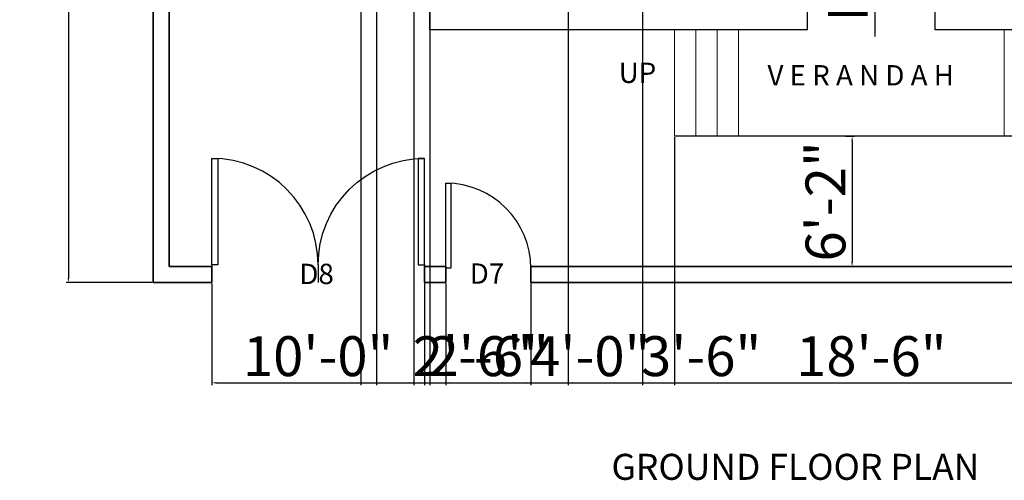
# Model space of a CAD drawing. Units: inches. Extents: x 164 to 1038, y 98 to 1358.
# Tile 1 of 4: x 199 to 754, y 98 to 358. Entities that reach past the tile are written whole.
import ezdxf

# ---------------------------------------------------------------- set-up
doc = ezdxf.new("R2010")
doc.units = ezdxf.units.IN
for name, color, linetype, lineweight in [('A-ANNO-DIMS', 7, 'Continuous', 18), ('A-ANNO-TEXT', 3, 'Continuous', 18), ('A-ANNO-TITL', 7, 'Continuous', 35), ('A-AREA-IDEN', 3, 'Continuous', 18), ('A-FLOR', 7, 'Continuous', 25), ('C-SITE-GATE', 6, 'Continuous', 25), ('C-SITE-WALL', 7, 'Continuous', 35), ('staircase', 4, 'Continuous', 18), ('wall', 7, 'Continuous', 35)]:
    doc.layers.add(name, color=color, linetype=linetype, lineweight=lineweight)
doc.styles.get("Standard").update_dxf_attribs({"font": 'arial.ttf'})
doc.dimstyles.new('ISO-25', dxfattribs={"dimtxt": 22.5, "dimasz": 2.5, "dimexe": 1.25, "dimexo": 0.625, "dimtad": 1, "dimdec": 0, "dimlunit": 3, "dimtxsty": 'Standard', "dimcen": 2.5, "dimadec": 0, "dimazin": 0, "dimtfac": 1, "dimtdec": 0, "dimtmove": 0, "dimatfit": 3, "dimfxl": 1, "dimarcsym": 0})

# ---------------------------------------------------------------- blocks, each defined once
blk = doc.blocks.new('*U3')
for p, q in [((0, 0), (0, -5)), ((30, 0), (30, -5))]:
    blk.add_line(p, q)
blk.add_lwpolyline([(0, 0), (0, 30), (1.75, 30), (1.75, 0)], close=True)
blk.add_arc((0, 0), 30, 0, 90)
blk = doc.blocks.new('*D20')
at = {"layer": 'A-ANNO-DIMS', "color": 0, "lineweight": -2, "transparency": 16777216}
for p, q in [((273.44, 1145.87), (224.94, 1145.87)), ((226.19, 1143.37), (226.19, 212.37)), ((273.44, 209.87), (224.94, 209.87))]:
    blk.add_line(p, q, dxfattribs=at)
at = {"layer": 'A-ANNO-DIMS', "color": 0, "transparency": 16777216}
for points in [[(225.78, 1143.37), (226.61, 1143.37), (226.19, 1145.87)], [(225.78, 212.37), (226.61, 212.37), (226.19, 209.87)]]:
    blk.add_solid(points, dxfattribs=at)
at = {"layer": 'Defpoints', "color": 0, "transparency": 16777216}
for p in [(274.07, 1145.87), (226.19, 209.87), (274.07, 209.87)]:
    blk.add_point(p, dxfattribs=at)
at = {"layer": 'A-ANNO-DIMS', "color": 0, "transparency": 16777216, "insert": (214.08, 677.87), "char_height": 22.5, "attachment_point": 5, "rotation": 90}
blk.add_mtext("78'", dxfattribs=at)
blk = doc.blocks.new('*D26')
at = {"layer": 'A-ANNO-DIMS', "color": 0, "lineweight": -2, "transparency": 16777216}
for p, q in [((664.43, 292.37), (669.48, 292.37)), ((668.23, 289.87), (668.23, 221.37)), ((664.43, 218.87), (669.48, 218.87))]:
    blk.add_line(p, q, dxfattribs=at)
at = {"layer": 'A-ANNO-DIMS', "color": 0, "transparency": 16777216}
for points in [[(667.81, 289.87), (668.65, 289.87), (668.23, 292.37)], [(667.81, 221.37), (668.65, 221.37), (668.23, 218.87)]]:
    blk.add_solid(points, dxfattribs=at)
at = {"layer": 'Defpoints', "color": 0, "transparency": 16777216}
for p in [(663.81, 292.37), (663.81, 218.87), (668.23, 218.87)]:
    blk.add_point(p, dxfattribs=at)
at = {"layer": 'A-ANNO-DIMS', "color": 0, "transparency": 16777216, "insert": (656.12, 255.62), "char_height": 22.5, "attachment_point": 5, "rotation": 90}
blk.add_mtext('6\'-2"', dxfattribs=at)
blk = doc.blocks.new('*D44')
at = {"layer": 'A-ANNO-DIMS', "color": 0, "lineweight": -2, "transparency": 16777216}
for p, q in [((677.56, 658.58), (682.23, 658.58)), ((680.98, 656.08), (680.98, 634.08)), ((677.56, 631.58), (682.23, 631.58)), ((680.98, 631.58), (680.98, 348.63))]:
    blk.add_line(p, q, dxfattribs=at)
at = {"layer": 'A-ANNO-DIMS', "color": 0, "transparency": 16777216}
for points in [[(680.57, 656.08), (681.4, 656.08), (680.98, 658.58)], [(680.57, 634.08), (681.4, 634.08), (680.98, 631.58)]]:
    blk.add_solid(points, dxfattribs=at)
at = {"layer": 'Defpoints', "color": 0, "transparency": 16777216}
for p in [(676.93, 658.58), (676.93, 631.58), (680.98, 631.58)]:
    blk.add_point(p, dxfattribs=at)
at = {"layer": 'A-ANNO-DIMS', "color": 0, "transparency": 16777216, "insert": (668.71, 488.85), "char_height": 22.5, "attachment_point": 5, "rotation": 90}
blk.add_mtext('ROCKER 2\'-3" TYP.', dxfattribs=at)
blk = doc.blocks.new('*D52')
at = {"layer": 'A-ANNO-DIMS', "color": 0, "lineweight": -2, "transparency": 16777216}
for p, q in [((307.07, 209.24), (307.07, 152.07)), ((427.07, 209.24), (427.07, 152.07)), ((309.57, 153.32), (424.57, 153.32))]:
    blk.add_line(p, q, dxfattribs=at)
at = {"layer": 'A-ANNO-DIMS', "color": 0, "transparency": 16777216}
for points in [[(309.57, 153.73), (309.57, 152.9), (307.07, 153.32)], [(424.57, 153.73), (424.57, 152.9), (427.07, 153.32)]]:
    blk.add_solid(points, dxfattribs=at)
at = {"layer": 'Defpoints', "color": 0, "transparency": 16777216}
for p in [(307.07, 209.87), (427.07, 209.87), (427.07, 153.32)]:
    blk.add_point(p, dxfattribs=at)
at = {"layer": 'A-ANNO-DIMS', "color": 0, "transparency": 16777216, "insert": (367.07, 165.43), "char_height": 22.5, "attachment_point": 5}
blk.add_mtext('10\'-0"', dxfattribs=at)
blk = doc.blocks.new('*D53')
at = {"layer": 'A-ANNO-DIMS', "color": 0, "lineweight": -2, "transparency": 16777216}
for p, q in [((439.07, 209.24), (439.07, 152.07)), ((487.07, 209.24), (487.07, 152.07)), ((441.57, 153.32), (484.57, 153.32)), ((487.07, 153.32), (551.53, 153.32))]:
    blk.add_line(p, q, dxfattribs=at)
at = {"layer": 'A-ANNO-DIMS', "color": 0, "transparency": 16777216}
for points in [[(441.57, 153.73), (441.57, 152.9), (439.07, 153.32)], [(484.57, 153.73), (484.57, 152.9), (487.07, 153.32)]]:
    blk.add_solid(points, dxfattribs=at)
at = {"layer": 'Defpoints', "color": 0, "transparency": 16777216}
for p in [(439.07, 209.87), (487.07, 209.87), (487.07, 153.32)]:
    blk.add_point(p, dxfattribs=at)
at = {"layer": 'A-ANNO-DIMS', "color": 0, "transparency": 16777216, "insert": (520.55, 165.43), "char_height": 22.5, "attachment_point": 5}
blk.add_mtext('4\'-0"', dxfattribs=at)
blk = doc.blocks.new('*D54')
at = {"layer": 'A-ANNO-DIMS', "color": 0, "lineweight": -2, "transparency": 16777216}
for p, q in [((391.07, 1028.24), (391.07, 152.07)), ((421.07, 1028.24), (421.07, 152.07)), ((393.57, 153.32), (418.57, 153.32)), ((421.07, 153.32), (485.01, 153.32))]:
    blk.add_line(p, q, dxfattribs=at)
at = {"layer": 'A-ANNO-DIMS', "color": 0, "transparency": 16777216}
for points in [[(393.57, 153.73), (393.57, 152.9), (391.07, 153.32)], [(418.57, 153.73), (418.57, 152.9), (421.07, 153.32)]]:
    blk.add_solid(points, dxfattribs=at)
at = {"layer": 'Defpoints', "color": 0, "transparency": 16777216}
for p in [(391.07, 1028.87), (421.07, 1028.87), (421.07, 153.32)]:
    blk.add_point(p, dxfattribs=at)
at = {"layer": 'A-ANNO-DIMS', "color": 0, "transparency": 16777216, "insert": (454.29, 165.43), "char_height": 22.5, "attachment_point": 5}
blk.add_mtext('2\'-6"', dxfattribs=at)
blk = doc.blocks.new('*D55')
at = {"layer": 'A-ANNO-DIMS', "color": 0, "lineweight": -2, "transparency": 16777216}
for p, q in [((508.07, 662.24), (508.07, 152.07)), ((550.07, 662.24), (550.07, 152.07)), ((510.57, 153.32), (547.57, 153.32)), ((550.07, 153.32), (613.61, 153.32))]:
    blk.add_line(p, q, dxfattribs=at)
at = {"layer": 'A-ANNO-DIMS', "color": 0, "transparency": 16777216}
for points in [[(510.57, 153.73), (510.57, 152.9), (508.07, 153.32)], [(547.57, 153.73), (547.57, 152.9), (550.07, 153.32)]]:
    blk.add_solid(points, dxfattribs=at)
at = {"layer": 'Defpoints', "color": 0, "transparency": 16777216}
for p in [(508.07, 662.87), (550.07, 662.87), (550.07, 153.32)]:
    blk.add_point(p, dxfattribs=at)
at = {"layer": 'A-ANNO-DIMS', "color": 0, "transparency": 16777216, "insert": (583.09, 165.44), "char_height": 22.5, "attachment_point": 5}
blk.add_mtext('3\'-6"', dxfattribs=at)
blk = doc.blocks.new('*D57')
at = {"layer": 'A-ANNO-DIMS', "color": 0, "lineweight": -2, "transparency": 16777216}
for p, q in [((400.07, 599.24), (400.07, 152.07)), ((430.07, 599.24), (430.07, 152.07)), ((402.57, 153.32), (427.57, 153.32)), ((430.07, 153.32), (494.01, 153.32))]:
    blk.add_line(p, q, dxfattribs=at)
at = {"layer": 'A-ANNO-DIMS', "color": 0, "transparency": 16777216}
for points in [[(402.57, 153.73), (402.57, 152.9), (400.07, 153.32)], [(427.57, 153.73), (427.57, 152.9), (430.07, 153.32)]]:
    blk.add_solid(points, dxfattribs=at)
at = {"layer": 'Defpoints', "color": 0, "transparency": 16777216}
for p in [(400.07, 599.87), (430.07, 599.87), (430.07, 153.32)]:
    blk.add_point(p, dxfattribs=at)
at = {"layer": 'A-ANNO-DIMS', "color": 0, "transparency": 16777216, "insert": (463.29, 165.43), "char_height": 22.5, "attachment_point": 5}
blk.add_mtext('2\'-6"', dxfattribs=at)
blk = doc.blocks.new('*D60')
at = {"layer": 'A-ANNO-DIMS', "color": 0, "lineweight": -2, "transparency": 16777216}
for p, q in [((568.07, 291.74), (568.07, 152.07)), ((790.07, 291.74), (790.07, 152.07)), ((570.57, 153.32), (787.57, 153.32))]:
    blk.add_line(p, q, dxfattribs=at)
at = {"layer": 'A-ANNO-DIMS', "color": 0, "transparency": 16777216}
for points in [[(570.57, 153.73), (570.57, 152.9), (568.07, 153.32)], [(787.57, 153.73), (787.57, 152.9), (790.07, 153.32)]]:
    blk.add_solid(points, dxfattribs=at)
at = {"layer": 'Defpoints', "color": 0, "transparency": 16777216}
for p in [(568.07, 292.37), (790.07, 292.37), (790.07, 153.32)]:
    blk.add_point(p, dxfattribs=at)
at = {"layer": 'A-ANNO-DIMS', "color": 0, "transparency": 16777216, "insert": (679.07, 165.43), "char_height": 22.5, "attachment_point": 5}
blk.add_mtext('18\'-6"', dxfattribs=at)

msp = doc.modelspace()

# ---------------------------------------------------------------- linework, layer by layer
at = {"layer": 'A-FLOR'}
for p, q in [((643.07, 352.37), (643.07, 388.37)), ((715.07, 352.37), (715.07, 388.37)), ((643.07, 352.37), (430.07, 352.37)), ((928.07, 352.37), (715.07, 352.37)), ((790.07, 292.37), (568.07, 292.37))]:
    msp.add_line(p, q, dxfattribs=at)
at = {"layer": 'C-SITE-WALL'}
for p, q in [((274.07, 1145.87), (274.07, 209.87)), ((283.07, 662.87), (283.07, 218.87)), ((307.07, 218.87), (283.07, 218.87)), ((307.07, 218.87), (307.07, 209.87)), ((427.07, 218.87), (427.07, 209.87)), ((439.07, 218.87), (427.07, 218.87)), ((439.07, 218.87), (439.07, 209.87)), ((487.07, 218.87), (487.07, 209.87)), ((832.07, 218.87), (487.07, 218.87)), ((307.07, 209.87), (274.07, 209.87)), ((439.07, 209.87), (427.07, 209.87)), ((832.07, 209.87), (487.07, 209.87))]:
    msp.add_line(p, q, dxfattribs=at)
at = {"layer": 'staircase'}
for p, q in [((568.07, 352.37), (568.07, 292.37)), ((580.07, 352.37), (580.07, 292.37)), ((592.07, 352.37), (592.07, 292.37)), ((604.07, 352.37), (604.07, 292.37)), ((754.07, 352.37), (754.07, 292.37))]:
    msp.add_line(p, q, dxfattribs=at)
at = {"layer": 'wall'}
msp.add_line((430.07, 626.87), (430.07, 352.37), dxfattribs=at)

# ---------------------------------------------------------------- block references
at = {"layer": 'C-SITE-GATE'}
for p, xscale, yscale, zscale in [((307.07, 219.87), 2, 2, 2), ((427.07, 219.87), -2, 2, 2), ((439.07, 217.87), 1.599999999999999, 1.599999999999999, 1.599999999999999)]:
    msp.add_blockref('*U3', p, dxfattribs=dict(at, xscale=xscale, yscale=yscale, zscale=zscale))

# ---------------------------------------------------------------- texts
at = {"layer": 'A-ANNO-TEXT'}
for s, p in [('UP', (536.58, 322.37)), ('D8', (356.48, 208.99)), ('D7', (452.58, 209.18))]:
    msp.add_text(s, height=11.466, dxfattribs=at).set_placement(p)
at = {"layer": 'A-ANNO-TITL'}
msp.add_text('GROUND FLOOR PLAN', height=14.6743, dxfattribs=at).set_placement((532.47, 98.62))
at = {"layer": 'A-AREA-IDEN'}
msp.add_text('V E R A N D A H', height=11.4664, dxfattribs=at).set_placement((620.5, 320.96))

# ---------------------------------------------------------------- dimensions: what is measured, and where the dimension line sits
at = {"layer": 'A-ANNO-DIMS'}
for base, p1, p2, picture, middle in [((226.19, 209.87), (274.07, 1145.87), (274.07, 209.87), '*D20', (214.08, 677.87)), ((668.23079344, 218.86625341), (663.80879534, 292.36625341), (663.80879534, 218.86625341), '*D26', (656.11790121, 255.61625341))]:
    dim = msp.add_linear_dim(base=base, p1=p1, p2=p2, angle=90, dimstyle='ISO-25', override={"dimclrd": 0, "dimclre": 0, "dimclrt": 0}, dxfattribs=at)
    dim.commit()
    dim.dimension.update_dxf_attribs({"geometry": picture, "text_midpoint": middle})
for base, p1, p2, picture, middle in [((421.07, 153.32), (391.07, 1028.87), (421.07, 1028.87), '*D54', (454.29, 165.43)), ((550.07, 153.32), (508.07, 662.87), (550.07, 662.87), '*D55', (583.09, 165.44)), ((430.07, 153.32), (400.07, 599.87), (430.07, 599.87), '*D57', (463.29, 165.43)), ((790.07, 153.32), (568.07, 292.37), (790.07, 292.37), '*D60', (679.07, 165.43)), ((427.07, 153.32), (307.07, 209.87), (427.07, 209.87), '*D52', (367.07, 165.43)), ((487.07, 153.32), (439.07, 209.87), (487.07, 209.87), '*D53', (520.55, 165.43))]:
    dim = msp.add_linear_dim(base=base, p1=p1, p2=p2, dimstyle='ISO-25', override={"dimdec": 1, "dimlfac": 1, "dimrnd": 0, "dimzin": 1, "dimdsep": 46, "dimlunit": 4, "dimfrac": 2}, dxfattribs=at)
    dim.commit()
    dim.dimension.update_dxf_attribs({"geometry": picture, "text_midpoint": middle})
dim = msp.add_linear_dim(base=(680.98, 631.58), p1=(676.93, 658.58), p2=(676.93, 631.58), angle=270, text='ROCKER <> TYP.', dimstyle='ISO-25', override={"dimdec": 1, "dimlfac": 1, "dimrnd": 0, "dimzin": 1, "dimdsep": 46, "dimlunit": 4, "dimfrac": 2}, dxfattribs=at)
dim.commit()
dim.dimension.update_dxf_attribs({"geometry": '*D44', "text_midpoint": (668.71, 488.85)})

doc.saveas('drawing.dxf')
